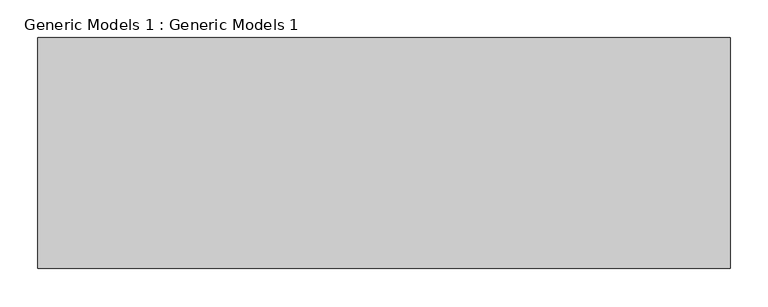
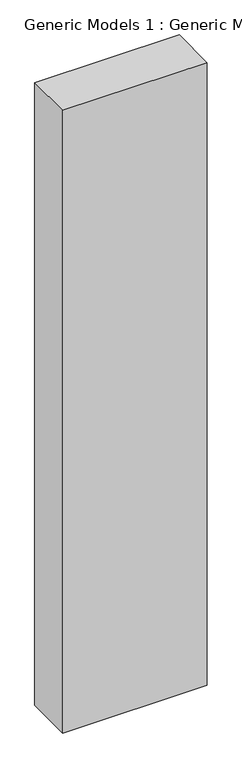
"""IFC4 building model written with IfcOpenShell, lengths in millimetres: proxy geometry, Generic Models 1 : Generic Models 1."""

from ifc_helpers import new_model, si_unit, frame, origin, place, context, project, spatial, polyline, outline, extrude, source, transform, mapped, element, save


def generic_models_1_generic_models_1_e82ef2ba(model_context):
    return source(origin(), model_context, "Body", "SweptSolid", [
        extrude(outline(polyline([(-4767.1906521, -11839.7310793), (-5681.5906521, -11839.7310793), (-5681.5906521, -11534.9310793), (-4767.1906521, -11534.9310793), (-4767.1906521, -11839.7310793)])), frame((0.0, 0.0, 76.2), z_axis=(0.0, 0.0, 1.0), x_axis=(1.0, 0.0, 0.0)), (0.0, 0.0, 1.0), 4162.6066296),
    ])


if __name__ == "__main__":
    model = new_model("IFC4")
    model_context = context("Model", 3, world=origin())
    ifc_project = project(units=[si_unit("LENGTHUNIT", "METRE", prefix="MILLI")], contexts=[model_context])
    site = spatial("IfcSite", under=ifc_project)
    building = spatial("IfcBuilding", under=site)
    placement = place(None, origin())
    generic_models_1_generic_models_1_shape = generic_models_1_generic_models_1_e82ef2ba(model_context)
    element("IfcBuildingElementProxy", 1, Name="Generic Models 1 : Generic Models 1", ObjectType="Generic Models 1 : Generic Models 1", at=placement, inside=building, context=model_context, shape_type="MappedRepresentation", body=[
        mapped(generic_models_1_generic_models_1_shape, transform((0.0, 0.0, 0.0), x_axis=(1.0, 0.0, 0.0), y_axis=(0.0, 1.0, 0.0), z_axis=(0.0, 0.0, 1.0))),
    ])
    save(model, "model.ifc")

# Revit data of these elements
# Element 1 (IfcBuildingElementProxy, "Generic Models 1 : Generic Models 1")
#   Materials on its faces: "GREY COLOUR FRAME"
# Materials
#   "GREY COLOUR FRAME": class "Generic", colour RGB 120 120 120, transparency 0, Cost = 0
